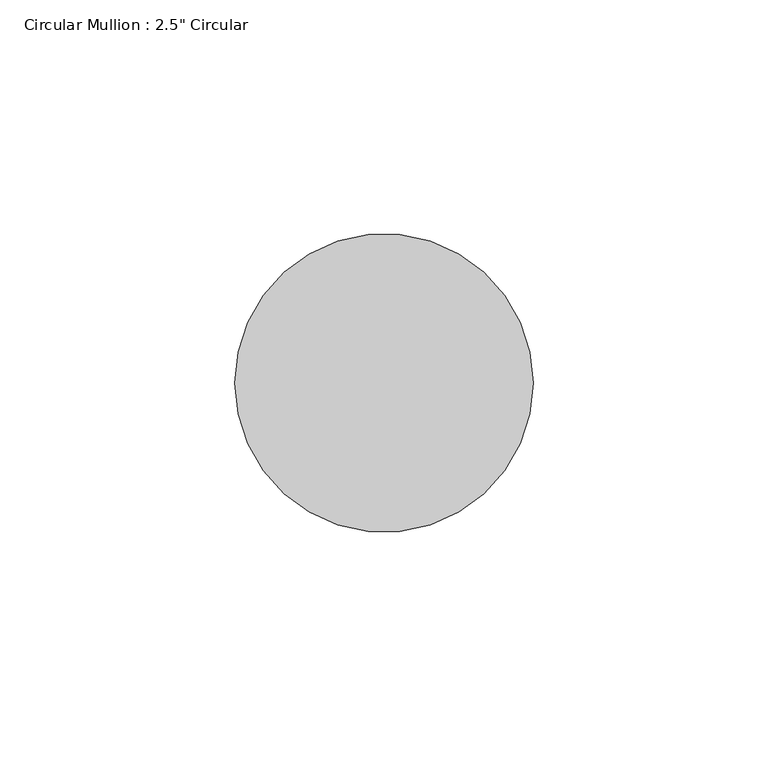
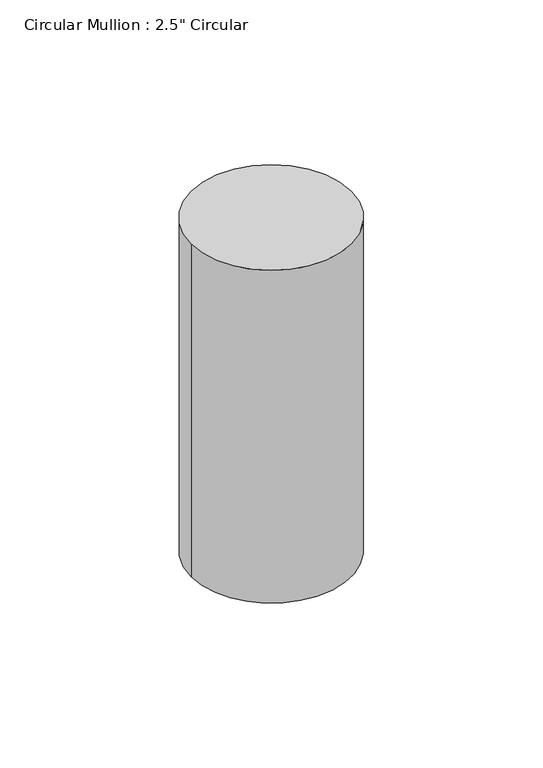
"""IFC4 building model written with IfcOpenShell, lengths in millimetres: member geometry."""

from ifc_helpers import new_model, si_unit, point, frame, origin, origin_2d, place, context, project, spatial, circle_curve, trimmed, segment, composite_curve, outline, extrude, source, transform, mapped, element, save


def member_e49bab3c(model_context):
    return source(origin(), model_context, "Body", "SweptSolid", [
        extrude(outline(composite_curve([segment(trimmed(circle_curve(origin_2d(), 31.75), [point((31.75, 0.0))], [point((-31.75, 0.0))], False, "CARTESIAN"), True, "CONTINUOUS"), segment(trimmed(circle_curve(origin_2d(), 31.75), [point((-31.75, 0.0))], [point((31.75, 0.0))], False, "CARTESIAN"), True, "CONTINUOUS")], self_intersect=False)), frame((0.0, 0.0, -139.7), z_axis=(0.0, 0.0, 1.0), x_axis=(1.0, 0.0, 0.0)), (0.0, 0.0, 1.0), 139.7),
    ])


if __name__ == "__main__":
    model = new_model("IFC4")
    model_context = context("Model", 3, world=origin())
    ifc_project = project(units=[si_unit("LENGTHUNIT", "METRE", prefix="MILLI")], contexts=[model_context])
    site = spatial("IfcSite", under=ifc_project)
    building = spatial("IfcBuilding", under=site)
    placement = place(None, origin())
    member_shape = member_e49bab3c(model_context)
    element("IfcMember", 1, ObjectType="Circular Mullion : 2.5\" Circular", at=placement, inside=building, context=model_context, shape_type="MappedRepresentation", body=[
        mapped(member_shape, transform((0.0, 0.0, 0.0), x_axis=(1.0, 0.0, 0.0), y_axis=(0.0, 1.0, 0.0), z_axis=(0.0, 0.0, 1.0))),
    ])
    save(model, "model.ifc")

# Revit data of these elements
# Type "Circular Mullion : 2.5\" Circular"
#   built-in parameter 1007350 = 0.104167 (stored number, unit not read)
# Element 1 (IfcMember, "Circular Mullion : 2.5\" Circular")
#   Materials on its faces: "Door - Frame"
# Materials
#   "Door - Frame": colour RGB 118 70 51, transparency 0, Cost = 0
